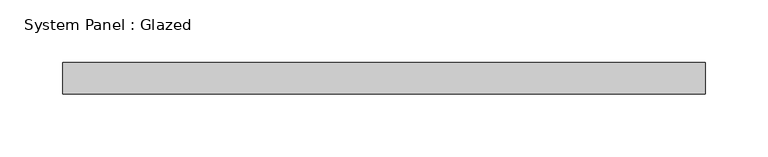
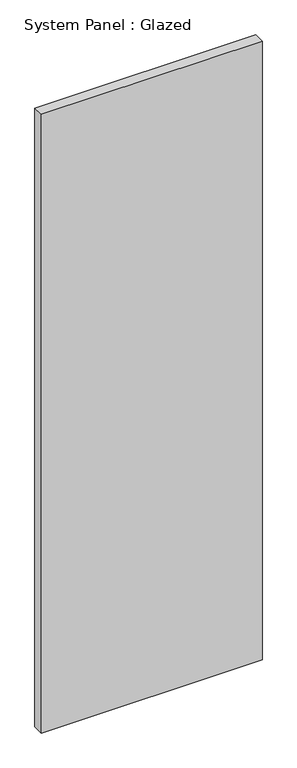
"""IFC4 building model written with IfcOpenShell, lengths in millimetres: plate geometry, System Panel : Glazed."""

from ifc_helpers import new_model, si_unit, origin, origin_with_axes, place, context, project, spatial, polyline, outline, extrude, source, transform, mapped, element, save


def system_panel_glazed_7a35cff4(model_context):
    return source(origin(), model_context, "Body", "SweptSolid", [
        extrude(outline(polyline([(257.175, 19.05), (-257.175, 19.05), (-257.175, 44.45), (257.175, 44.45), (257.175, 19.05)])), origin_with_axes(), (0.0, 0.0, 1.0), 1524.0),
    ])


if __name__ == "__main__":
    model = new_model("IFC4")
    model_context = context("Model", 3, world=origin())
    ifc_project = project(units=[si_unit("LENGTHUNIT", "METRE", prefix="MILLI")], contexts=[model_context])
    site = spatial("IfcSite", under=ifc_project)
    building = spatial("IfcBuilding", under=site)
    placement = place(None, origin())
    system_panel_glazed_shape = system_panel_glazed_7a35cff4(model_context)
    element("IfcPlate", 1, ObjectType="System Panel : Glazed", at=placement, inside=building, context=model_context, shape_type="MappedRepresentation", body=[
        mapped(system_panel_glazed_shape, transform((0.0, 0.0, 0.0), x_axis=(1.0, 0.0, 0.0), y_axis=(0.0, 1.0, 0.0), z_axis=(0.0, 0.0, 1.0))),
    ])
    save(model, "model.ifc")

# Revit data of these elements
# Type "System Panel : Glazed"
#   Construction Type Id = "GSP4R"
#   Analytic Construction = "1/8 in Pilkington single glazing"
#   Visual Light Transmittance = 0.9
#   Solar Heat Gain Coefficient = 0.86
#   Heat Transfer Coefficient (U) = 1.18115 BTU/(h·ft²·°F)
#   Define Thermal Properties by = 1
# Element 1 (IfcPlate, "System Panel : Glazed")
#   Materials on its faces: "Glass"
# Materials
#   "Glass": class "Glass", colour RGB 0 128 192, transparency 0.75, Description = "Soda Lime Glass", Cost = 0
